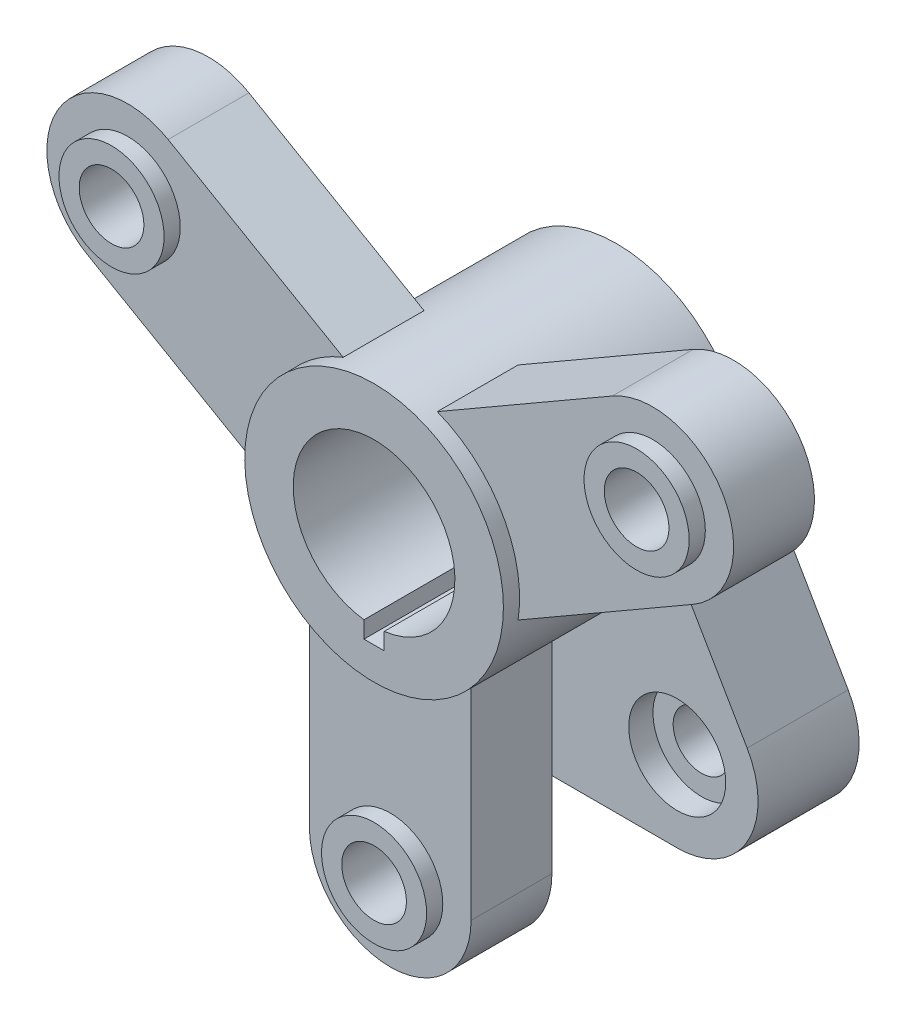
ISO-10303-21;
HEADER;
FILE_DESCRIPTION(('STEP AP214'),'2;1');
FILE_NAME('part.step','',(''),(''),'','','');
FILE_SCHEMA(('AUTOMOTIVE_DESIGN { 1 0 10303 214 1 1 1 1 }'));
ENDSEC;
DATA;
#1=APPLICATION_CONTEXT('core data for automotive mechanical design processes');
#2=APPLICATION_PROTOCOL_DEFINITION('international standard','automotive_design',2000,#1);
#3=PRODUCT_CONTEXT('',#1,'mechanical');
#4=PRODUCT('Part','Part','',(#3));
#5=PRODUCT_RELATED_PRODUCT_CATEGORY('part','',(#4));
#6=PRODUCT_DEFINITION_FORMATION('','',#4);
#7=PRODUCT_DEFINITION_CONTEXT('part definition',#1,'design');
#8=PRODUCT_DEFINITION('design','',#6,#7);
#9=PRODUCT_DEFINITION_SHAPE('','',#8);
#10=(LENGTH_UNIT() NAMED_UNIT(*) SI_UNIT(.MILLI.,.METRE.));
#11=(NAMED_UNIT(*) PLANE_ANGLE_UNIT() SI_UNIT($,.RADIAN.));
#12=(NAMED_UNIT(*) SI_UNIT($,.STERADIAN.) SOLID_ANGLE_UNIT());
#13=UNCERTAINTY_MEASURE_WITH_UNIT(LENGTH_MEASURE(1.E-05),#10,'distance_accuracy_value','');
#14=(GEOMETRIC_REPRESENTATION_CONTEXT(3) GLOBAL_UNCERTAINTY_ASSIGNED_CONTEXT((#13)) GLOBAL_UNIT_ASSIGNED_CONTEXT((#10,
#11,#12)) REPRESENTATION_CONTEXT('',''));
#15=CARTESIAN_POINT('',(0.,0.,0.));
#16=DIRECTION('',(0.,0.,1.));
#17=DIRECTION('',(1.,0.,0.));
#18=AXIS2_PLACEMENT_3D('',#15,#16,#17);
#19=CARTESIAN_POINT('',(0.,0.,56.));
#20=DIRECTION('',(0.,0.,1.));
#21=DIRECTION('',(1.,0.,0.));
#22=AXIS2_PLACEMENT_3D('',#19,#20,#21);
#23=PLANE('',#22);
#24=CARTESIAN_POINT('',(-64.951905283833,37.4999999999998,56.));
#25=DIRECTION('',(0.,0.,1.));
#26=DIRECTION('',(1.,0.,0.));
#27=AXIS2_PLACEMENT_3D('',#24,#25,#26);
#28=CIRCLE('',#27,13.);
#29=CARTESIAN_POINT('',(-51.951905283833,37.4999999999998,56.));
#30=VERTEX_POINT('',#29);
#31=EDGE_CURVE('E262',#30,#30,#28,.T.);
#32=ORIENTED_EDGE('',*,*,#31,.F.);
#33=EDGE_LOOP('',(#32));
#34=FACE_BOUND('',#33,.T.);
#35=CARTESIAN_POINT('',(0.,0.,56.));
#36=DIRECTION('',(0.,0.,1.));
#37=DIRECTION('',(1.,0.,0.));
#38=AXIS2_PLACEMENT_3D('',#35,#36,#37);
#39=CIRCLE('',#38,32.);
#40=CARTESIAN_POINT('',(-11.633307652784,29.8105040724855,56.));
#41=VERTEX_POINT('',#40);
#42=CARTESIAN_POINT('',(-31.6333076527839,-4.83051207889205,56.));
#43=VERTEX_POINT('',#42);
#44=EDGE_CURVE('E11',#41,#43,#39,.T.);
#45=ORIENTED_EDGE('',*,*,#44,.F.);
#46=DIRECTION('',(-0.86602540378444,0.499999999999998,0.));
#47=VECTOR('',#46,1.);
#48=CARTESIAN_POINT('',(-11.633307652784,29.8105040724855,56.));
#49=LINE('',#48,#47);
#50=CARTESIAN_POINT('',(-54.9519052838331,54.8205080756886,56.));
#51=VERTEX_POINT('',#50);
#52=EDGE_CURVE('E273',#41,#51,#49,.T.);
#53=ORIENTED_EDGE('',*,*,#52,.T.);
#54=CARTESIAN_POINT('',(-64.951905283833,37.4999999999998,56.));
#55=DIRECTION('',(0.,0.,1.));
#56=DIRECTION('',(1.,0.,0.));
#57=AXIS2_PLACEMENT_3D('',#54,#55,#56);
#58=CIRCLE('',#57,20.);
#59=CARTESIAN_POINT('',(-74.9519052838329,20.179491924311,56.));
#60=VERTEX_POINT('',#59);
#61=EDGE_CURVE('E295',#51,#60,#58,.T.);
#62=ORIENTED_EDGE('',*,*,#61,.T.);
#63=DIRECTION('',(0.86602540378444,-0.499999999999998,0.));
#64=VECTOR('',#63,1.);
#65=CARTESIAN_POINT('',(-31.6333076527839,-4.83051207889205,56.));
#66=LINE('',#65,#64);
#67=EDGE_CURVE('E278',#60,#43,#66,.T.);
#68=ORIENTED_EDGE('',*,*,#67,.T.);
#69=EDGE_LOOP('',(#45,#53,#62,#68));
#70=FACE_BOUND('',#69,.T.);
#71=ADVANCED_FACE('F50',(#34,#70),#23,.T.);
#72=CARTESIAN_POINT('',(0.,-75.,56.));
#73=DIRECTION('',(0.,0.,1.));
#74=DIRECTION('',(1.,0.,0.));
#75=AXIS2_PLACEMENT_3D('',#72,#73,#74);
#76=CIRCLE('',#75,13.);
#77=CARTESIAN_POINT('',(13.,-75.,56.));
#78=VERTEX_POINT('',#77);
#79=EDGE_CURVE('E255',#78,#78,#76,.T.);
#80=ORIENTED_EDGE('',*,*,#79,.F.);
#81=EDGE_LOOP('',(#80));
#82=FACE_BOUND('',#81,.T.);
#83=CARTESIAN_POINT('',(-20.,-24.9799919935936,56.));
#84=VERTEX_POINT('',#83);
#85=CARTESIAN_POINT('',(20.,-24.9799919935936,56.));
#86=VERTEX_POINT('',#85);
#87=EDGE_CURVE('E57',#84,#86,#39,.T.);
#88=ORIENTED_EDGE('',*,*,#87,.F.);
#89=DIRECTION('',(0.,-1.,0.));
#90=VECTOR('',#89,1.);
#91=CARTESIAN_POINT('',(-20.,-75.,56.));
#92=LINE('',#91,#90);
#93=CARTESIAN_POINT('',(-20.,-75.,56.));
#94=VERTEX_POINT('',#93);
#95=EDGE_CURVE('E297',#84,#94,#92,.T.);
#96=ORIENTED_EDGE('',*,*,#95,.T.);
#97=CARTESIAN_POINT('',(0.,-75.,56.));
#98=DIRECTION('',(0.,0.,1.));
#99=DIRECTION('',(1.,0.,0.));
#100=AXIS2_PLACEMENT_3D('',#97,#98,#99);
#101=CIRCLE('',#100,20.);
#102=CARTESIAN_POINT('',(20.,-75.,56.));
#103=VERTEX_POINT('',#102);
#104=EDGE_CURVE('E325',#94,#103,#101,.T.);
#105=ORIENTED_EDGE('',*,*,#104,.T.);
#106=DIRECTION('',(0.,1.,0.));
#107=VECTOR('',#106,1.);
#108=CARTESIAN_POINT('',(20.,-75.,56.));
#109=LINE('',#108,#107);
#110=EDGE_CURVE('E309',#103,#86,#109,.T.);
#111=ORIENTED_EDGE('',*,*,#110,.T.);
#112=EDGE_LOOP('',(#88,#96,#105,#111));
#113=FACE_BOUND('',#112,.T.);
#114=ADVANCED_FACE('F483',(#82,#113),#23,.T.);
#115=CARTESIAN_POINT('',(0.,-65.,25.));
#116=DIRECTION('',(0.,1.,0.));
#117=DIRECTION('',(0.,0.,1.));
#118=AXIS2_PLACEMENT_3D('',#115,#116,#117);
#119=PLANE('',#118);
#120=DIRECTION('',(1.,0.,0.));
#121=VECTOR('',#120,1.);
#122=CARTESIAN_POINT('',(0.,-65.,0.));
#123=LINE('',#122,#121);
#124=CARTESIAN_POINT('',(-40.,-65.,0.));
#125=VERTEX_POINT('',#124);
#126=CARTESIAN_POINT('',(40.,-65.,0.));
#127=VERTEX_POINT('',#126);
#128=EDGE_CURVE('E360',#125,#127,#123,.T.);
#129=ORIENTED_EDGE('',*,*,#128,.T.);
#130=DIRECTION('',(0.,0.,-1.));
#131=VECTOR('',#130,1.);
#132=CARTESIAN_POINT('',(40.,-65.,25.));
#133=LINE('',#132,#131);
#134=CARTESIAN_POINT('',(40.,-65.,25.));
#135=VERTEX_POINT('',#134);
#136=EDGE_CURVE('E366',#135,#127,#133,.T.);
#137=ORIENTED_EDGE('',*,*,#136,.F.);
#138=DIRECTION('',(1.,0.,0.));
#139=VECTOR('',#138,1.);
#140=CARTESIAN_POINT('',(0.,-65.,25.));
#141=LINE('',#140,#139);
#142=CARTESIAN_POINT('',(-40.,-65.,25.));
#143=VERTEX_POINT('',#142);
#144=EDGE_CURVE('E369',#143,#135,#141,.T.);
#145=ORIENTED_EDGE('',*,*,#144,.F.);
#146=DIRECTION('',(0.,0.,-1.));
#147=VECTOR('',#146,1.);
#148=CARTESIAN_POINT('',(-40.,-65.,25.));
#149=LINE('',#148,#147);
#150=EDGE_CURVE('E382',#143,#125,#149,.T.);
#151=ORIENTED_EDGE('',*,*,#150,.T.);
#152=EDGE_LOOP('',(#129,#137,#145,#151));
#153=FACE_BOUND('',#152,.T.);
#154=ADVANCED_FACE('F47',(#153),#119,.F.);
#155=CARTESIAN_POINT('',(40.,-45.,25.));
#156=DIRECTION('',(0.,0.,-1.));
#157=DIRECTION('',(-1.,0.,0.));
#158=AXIS2_PLACEMENT_3D('',#155,#156,#157);
#159=CYLINDRICAL_SURFACE('',#158,20.);
#160=CARTESIAN_POINT('',(40.,-45.,0.));
#161=DIRECTION('',(0.,0.,1.));
#162=DIRECTION('',(1.,0.,0.));
#163=AXIS2_PLACEMENT_3D('',#160,#161,#162);
#164=CIRCLE('',#163,20.);
#165=CARTESIAN_POINT('',(57.2965517241379,-34.9586206896552,0.));
#166=VERTEX_POINT('',#165);
#167=EDGE_CURVE('E387',#127,#166,#164,.T.);
#168=ORIENTED_EDGE('',*,*,#167,.T.);
#169=DIRECTION('',(0.,0.,-1.));
#170=VECTOR('',#169,1.);
#171=CARTESIAN_POINT('',(57.2965517241379,-34.9586206896552,25.));
#172=LINE('',#171,#170);
#173=CARTESIAN_POINT('',(57.2965517241379,-34.9586206896552,25.));
#174=VERTEX_POINT('',#173);
#175=EDGE_CURVE('E410',#174,#166,#172,.T.);
#176=ORIENTED_EDGE('',*,*,#175,.F.);
#177=CARTESIAN_POINT('',(40.,-45.,25.));
#178=DIRECTION('',(0.,0.,1.));
#179=DIRECTION('',(1.,0.,0.));
#180=AXIS2_PLACEMENT_3D('',#177,#178,#179);
#181=CIRCLE('',#180,20.);
#182=EDGE_CURVE('E375',#135,#174,#181,.T.);
#183=ORIENTED_EDGE('',*,*,#182,.F.);
#184=ORIENTED_EDGE('',*,*,#136,.T.);
#185=EDGE_LOOP('',(#168,#176,#183,#184));
#186=FACE_BOUND('',#185,.T.);
#187=ADVANCED_FACE('F467',(#186),#159,.T.);
#188=CARTESIAN_POINT('',(27.6744827586207,16.0662068965517,25.));
#189=DIRECTION('',(0.864827586206897,0.502068965517242,0.));
#190=DIRECTION('',(-0.502068965517242,0.864827586206897,0.));
#191=AXIS2_PLACEMENT_3D('',#188,#189,#190);
#192=PLANE('',#191);
#193=DIRECTION('',(0.502068965517242,-0.864827586206896,0.));
#194=VECTOR('',#193,1.);
#195=CARTESIAN_POINT('',(27.6744827586207,16.0662068965517,0.));
#196=LINE('',#195,#194);
#197=CARTESIAN_POINT('',(27.6744827586207,16.0662068965517,0.));
#198=VERTEX_POINT('',#197);
#199=EDGE_CURVE('E386',#198,#166,#196,.T.);
#200=ORIENTED_EDGE('',*,*,#199,.F.);
#201=DIRECTION('',(0.,0.,-1.));
#202=VECTOR('',#201,1.);
#203=CARTESIAN_POINT('',(27.6744827586207,16.0662068965517,25.));
#204=LINE('',#203,#202);
#205=CARTESIAN_POINT('',(27.6744827586207,16.0662068965517,25.));
#206=VERTEX_POINT('',#205);
#207=EDGE_CURVE('E403',#206,#198,#204,.T.);
#208=ORIENTED_EDGE('',*,*,#207,.F.);
#209=DIRECTION('',(0.502068965517242,-0.864827586206896,0.));
#210=VECTOR('',#209,1.);
#211=CARTESIAN_POINT('',(27.6744827586207,16.0662068965517,25.));
#212=LINE('',#211,#210);
#213=EDGE_CURVE('E374',#206,#174,#212,.T.);
#214=ORIENTED_EDGE('',*,*,#213,.T.);
#215=ORIENTED_EDGE('',*,*,#175,.T.);
#216=EDGE_LOOP('',(#200,#208,#214,#215));
#217=FACE_BOUND('',#216,.T.);
#218=ADVANCED_FACE('F466',(#217),#192,.T.);
#219=CARTESIAN_POINT('',(0.,0.,25.));
#220=DIRECTION('',(0.,0.,-1.));
#221=DIRECTION('',(-1.,0.,0.));
#222=AXIS2_PLACEMENT_3D('',#219,#220,#221);
#223=CYLINDRICAL_SURFACE('',#222,32.);
#224=DIRECTION('',(0.,0.,1.));
#225=VECTOR('',#224,1.);
#226=CARTESIAN_POINT('',(-11.633307652784,29.8105040724855,36.));
#227=LINE('',#226,#225);
#228=CARTESIAN_POINT('',(-11.633307652784,29.8105040724855,36.));
#229=VERTEX_POINT('',#228);
#230=EDGE_CURVE('E286',#229,#41,#227,.T.);
#231=ORIENTED_EDGE('',*,*,#230,.T.);
#232=ORIENTED_EDGE('',*,*,#44,.T.);
#233=DIRECTION('',(0.,0.,1.));
#234=VECTOR('',#233,1.);
#235=CARTESIAN_POINT('',(-31.6333076527839,-4.83051207889205,36.));
#236=LINE('',#235,#234);
#237=CARTESIAN_POINT('',(-31.6333076527839,-4.83051207889205,36.));
#238=VERTEX_POINT('',#237);
#239=EDGE_CURVE('E298',#238,#43,#236,.T.);
#240=ORIENTED_EDGE('',*,*,#239,.F.);
#241=CARTESIAN_POINT('',(0.,0.,36.));
#242=DIRECTION('',(0.,0.,-1.));
#243=DIRECTION('',(1.,0.,0.));
#244=AXIS2_PLACEMENT_3D('',#241,#242,#243);
#245=CIRCLE('',#244,32.);
#246=EDGE_CURVE('E277',#238,#229,#245,.T.);
#247=ORIENTED_EDGE('',*,*,#246,.T.);
#248=EDGE_LOOP('',(#231,#232,#240,#247));
#249=FACE_BOUND('',#248,.T.);
#250=DIRECTION('',(0.,0.,1.));
#251=VECTOR('',#250,1.);
#252=CARTESIAN_POINT('',(-20.,-24.9799919935936,36.));
#253=LINE('',#252,#251);
#254=CARTESIAN_POINT('',(-20.,-24.9799919935936,36.));
#255=VERTEX_POINT('',#254);
#256=EDGE_CURVE('E317',#255,#84,#253,.T.);
#257=ORIENTED_EDGE('',*,*,#256,.T.);
#258=ORIENTED_EDGE('',*,*,#87,.T.);
#259=DIRECTION('',(0.,0.,1.));
#260=VECTOR('',#259,1.);
#261=CARTESIAN_POINT('',(20.,-24.9799919935936,36.));
#262=LINE('',#261,#260);
#263=CARTESIAN_POINT('',(20.,-24.9799919935936,36.));
#264=VERTEX_POINT('',#263);
#265=EDGE_CURVE('E326',#264,#86,#262,.T.);
#266=ORIENTED_EDGE('',*,*,#265,.F.);
#267=CARTESIAN_POINT('',(0.,0.,36.));
#268=DIRECTION('',(0.,0.,-1.));
#269=DIRECTION('',(1.,0.,0.));
#270=AXIS2_PLACEMENT_3D('',#267,#268,#269);
#271=CIRCLE('',#270,32.);
#272=EDGE_CURVE('E308',#264,#255,#271,.T.);
#273=ORIENTED_EDGE('',*,*,#272,.T.);
#274=EDGE_LOOP('',(#257,#258,#266,#273));
#275=FACE_BOUND('',#274,.T.);
#276=CARTESIAN_POINT('',(31.6314798513526,-4.84246656296924,56.));
#277=VERTEX_POINT('',#276);
#278=CARTESIAN_POINT('',(11.633307652784,29.8105040724856,56.));
#279=VERTEX_POINT('',#278);
#280=EDGE_CURVE('E59',#277,#279,#39,.T.);
#281=ORIENTED_EDGE('',*,*,#280,.T.);
#282=DIRECTION('',(0.,0.,1.));
#283=VECTOR('',#282,1.);
#284=CARTESIAN_POINT('',(11.633307652784,29.8105040724856,36.));
#285=LINE('',#284,#283);
#286=CARTESIAN_POINT('',(11.633307652784,29.8105040724856,36.));
#287=VERTEX_POINT('',#286);
#288=EDGE_CURVE('E354',#287,#279,#285,.T.);
#289=ORIENTED_EDGE('',*,*,#288,.F.);
#290=CARTESIAN_POINT('',(0.,0.,36.));
#291=DIRECTION('',(0.,0.,-1.));
#292=DIRECTION('',(1.,0.,0.));
#293=AXIS2_PLACEMENT_3D('',#290,#291,#292);
#294=CIRCLE('',#293,32.);
#295=CARTESIAN_POINT('',(31.6314798513526,-4.84246656296924,36.));
#296=VERTEX_POINT('',#295);
#297=EDGE_CURVE('E338',#287,#296,#294,.T.);
#298=ORIENTED_EDGE('',*,*,#297,.T.);
#299=DIRECTION('',(0.,0.,1.));
#300=VECTOR('',#299,1.);
#301=CARTESIAN_POINT('',(31.6314798513526,-4.84246656296924,36.));
#302=LINE('',#301,#300);
#303=EDGE_CURVE('E350',#296,#277,#302,.T.);
#304=ORIENTED_EDGE('',*,*,#303,.T.);
#305=EDGE_LOOP('',(#281,#289,#298,#304));
#306=FACE_BOUND('',#305,.T.);
#307=CARTESIAN_POINT('',(0.,0.,0.));
#308=DIRECTION('',(0.,0.,1.));
#309=DIRECTION('',(1.,0.,0.));
#310=AXIS2_PLACEMENT_3D('',#307,#308,#309);
#311=CIRCLE('',#310,32.);
#312=CARTESIAN_POINT('',(-27.6744827586207,16.0662068965517,0.));
#313=VERTEX_POINT('',#312);
#314=EDGE_CURVE('E395',#198,#313,#311,.T.);
#315=ORIENTED_EDGE('',*,*,#314,.T.);
#316=DIRECTION('',(0.,0.,-1.));
#317=VECTOR('',#316,1.);
#318=CARTESIAN_POINT('',(-27.6744827586207,16.0662068965517,25.));
#319=LINE('',#318,#317);
#320=CARTESIAN_POINT('',(-27.6744827586207,16.0662068965517,25.));
#321=VERTEX_POINT('',#320);
#322=EDGE_CURVE('E401',#321,#313,#319,.T.);
#323=ORIENTED_EDGE('',*,*,#322,.F.);
#324=CARTESIAN_POINT('',(0.,0.,25.));
#325=DIRECTION('',(0.,0.,1.));
#326=DIRECTION('',(1.,0.,0.));
#327=AXIS2_PLACEMENT_3D('',#324,#325,#326);
#328=CIRCLE('',#327,32.);
#329=EDGE_CURVE('E364',#321,#206,#328,.T.);
#330=ORIENTED_EDGE('',*,*,#329,.T.);
#331=ORIENTED_EDGE('',*,*,#207,.T.);
#332=EDGE_LOOP('',(#315,#323,#330,#331));
#333=FACE_BOUND('',#332,.T.);
#334=CARTESIAN_POINT('',(0.,0.,60.));
#335=DIRECTION('',(0.,0.,1.));
#336=DIRECTION('',(1.,0.,0.));
#337=AXIS2_PLACEMENT_3D('',#334,#335,#336);
#338=CIRCLE('',#337,32.);
#339=CARTESIAN_POINT('',(32.,0.,60.));
#340=VERTEX_POINT('',#339);
#341=EDGE_CURVE('E269',#340,#340,#338,.T.);
#342=ORIENTED_EDGE('',*,*,#341,.F.);
#343=EDGE_LOOP('',(#342));
#344=FACE_BOUND('',#343,.T.);
#345=ADVANCED_FACE('F449',(#249,#275,#306,#333,#344),#223,.T.);
#346=CARTESIAN_POINT('',(-27.6744827586207,16.0662068965517,25.));
#347=DIRECTION('',(-0.864827586206897,0.502068965517241,0.));
#348=DIRECTION('',(-0.502068965517241,-0.864827586206897,0.));
#349=AXIS2_PLACEMENT_3D('',#346,#347,#348);
#350=PLANE('',#349);
#351=DIRECTION('',(0.502068965517241,0.864827586206897,0.));
#352=VECTOR('',#351,1.);
#353=CARTESIAN_POINT('',(-27.6744827586207,16.0662068965517,0.));
#354=LINE('',#353,#352);
#355=CARTESIAN_POINT('',(-57.2965517241379,-34.9586206896552,0.));
#356=VERTEX_POINT('',#355);
#357=EDGE_CURVE('E394',#356,#313,#354,.T.);
#358=ORIENTED_EDGE('',*,*,#357,.F.);
#359=DIRECTION('',(0.,0.,-1.));
#360=VECTOR('',#359,1.);
#361=CARTESIAN_POINT('',(-57.2965517241379,-34.9586206896552,25.));
#362=LINE('',#361,#360);
#363=CARTESIAN_POINT('',(-57.2965517241379,-34.9586206896552,25.));
#364=VERTEX_POINT('',#363);
#365=EDGE_CURVE('E402',#364,#356,#362,.T.);
#366=ORIENTED_EDGE('',*,*,#365,.F.);
#367=DIRECTION('',(0.502068965517241,0.864827586206897,0.));
#368=VECTOR('',#367,1.);
#369=CARTESIAN_POINT('',(-27.6744827586207,16.0662068965517,25.));
#370=LINE('',#369,#368);
#371=EDGE_CURVE('E378',#364,#321,#370,.T.);
#372=ORIENTED_EDGE('',*,*,#371,.T.);
#373=ORIENTED_EDGE('',*,*,#322,.T.);
#374=EDGE_LOOP('',(#358,#366,#372,#373));
#375=FACE_BOUND('',#374,.T.);
#376=ADVANCED_FACE('F453',(#375),#350,.T.);
#377=CARTESIAN_POINT('',(-40.,-45.,25.));
#378=DIRECTION('',(0.,0.,-1.));
#379=DIRECTION('',(-1.,0.,0.));
#380=AXIS2_PLACEMENT_3D('',#377,#378,#379);
#381=CYLINDRICAL_SURFACE('',#380,20.);
#382=CARTESIAN_POINT('',(-40.,-45.,0.));
#383=DIRECTION('',(0.,0.,1.));
#384=DIRECTION('',(1.,0.,0.));
#385=AXIS2_PLACEMENT_3D('',#382,#383,#384);
#386=CIRCLE('',#385,20.);
#387=EDGE_CURVE('E373',#356,#125,#386,.T.);
#388=ORIENTED_EDGE('',*,*,#387,.T.);
#389=ORIENTED_EDGE('',*,*,#150,.F.);
#390=CARTESIAN_POINT('',(-40.,-45.,25.));
#391=DIRECTION('',(0.,0.,1.));
#392=DIRECTION('',(1.,0.,0.));
#393=AXIS2_PLACEMENT_3D('',#390,#391,#392);
#394=CIRCLE('',#393,20.);
#395=EDGE_CURVE('E381',#364,#143,#394,.T.);
#396=ORIENTED_EDGE('',*,*,#395,.F.);
#397=ORIENTED_EDGE('',*,*,#365,.T.);
#398=EDGE_LOOP('',(#388,#389,#396,#397));
#399=FACE_BOUND('',#398,.T.);
#400=ADVANCED_FACE('F444',(#399),#381,.T.);
#401=CARTESIAN_POINT('',(0.,0.,25.));
#402=DIRECTION('',(0.,0.,1.));
#403=DIRECTION('',(1.,0.,0.));
#404=AXIS2_PLACEMENT_3D('',#401,#402,#403);
#405=PLANE('',#404);
#406=CARTESIAN_POINT('',(-40.,-45.,25.));
#407=DIRECTION('',(0.,0.,1.));
#408=DIRECTION('',(1.,0.,0.));
#409=AXIS2_PLACEMENT_3D('',#406,#407,#408);
#410=CIRCLE('',#409,12.);
#411=CARTESIAN_POINT('',(-28.,-45.,25.));
#412=VERTEX_POINT('',#411);
#413=EDGE_CURVE('E428',#412,#412,#410,.T.);
#414=ORIENTED_EDGE('',*,*,#413,.F.);
#415=EDGE_LOOP('',(#414));
#416=FACE_BOUND('',#415,.T.);
#417=CARTESIAN_POINT('',(40.,-45.,25.));
#418=DIRECTION('',(0.,0.,1.));
#419=DIRECTION('',(1.,0.,0.));
#420=AXIS2_PLACEMENT_3D('',#417,#418,#419);
#421=CIRCLE('',#420,12.);
#422=CARTESIAN_POINT('',(52.,-45.,25.));
#423=VERTEX_POINT('',#422);
#424=EDGE_CURVE('E418',#423,#423,#421,.T.);
#425=ORIENTED_EDGE('',*,*,#424,.F.);
#426=EDGE_LOOP('',(#425));
#427=FACE_BOUND('',#426,.T.);
#428=ORIENTED_EDGE('',*,*,#329,.F.);
#429=ORIENTED_EDGE('',*,*,#371,.F.);
#430=ORIENTED_EDGE('',*,*,#395,.T.);
#431=ORIENTED_EDGE('',*,*,#144,.T.);
#432=ORIENTED_EDGE('',*,*,#182,.T.);
#433=ORIENTED_EDGE('',*,*,#213,.F.);
#434=EDGE_LOOP('',(#428,#429,#430,#431,#432,#433));
#435=FACE_BOUND('',#434,.T.);
#436=ADVANCED_FACE('F438',(#416,#427,#435),#405,.T.);
#437=CARTESIAN_POINT('',(0.,0.,0.));
#438=DIRECTION('',(0.,0.,1.));
#439=DIRECTION('',(1.,0.,0.));
#440=AXIS2_PLACEMENT_3D('',#437,#438,#439);
#441=PLANE('',#440);
#442=CARTESIAN_POINT('',(-40.,-45.,0.));
#443=DIRECTION('',(0.,0.,1.));
#444=DIRECTION('',(1.,0.,0.));
#445=AXIS2_PLACEMENT_3D('',#442,#443,#444);
#446=CIRCLE('',#445,7.);
#447=CARTESIAN_POINT('',(-33.,-45.,0.));
#448=VERTEX_POINT('',#447);
#449=EDGE_CURVE('E51',#448,#448,#446,.T.);
#450=ORIENTED_EDGE('',*,*,#449,.T.);
#451=EDGE_LOOP('',(#450));
#452=FACE_BOUND('',#451,.T.);
#453=CARTESIAN_POINT('',(40.,-45.,0.));
#454=DIRECTION('',(0.,0.,1.));
#455=DIRECTION('',(1.,0.,0.));
#456=AXIS2_PLACEMENT_3D('',#453,#454,#455);
#457=CIRCLE('',#456,7.);
#458=CARTESIAN_POINT('',(47.,-45.,0.));
#459=VERTEX_POINT('',#458);
#460=EDGE_CURVE('E409',#459,#459,#457,.T.);
#461=ORIENTED_EDGE('',*,*,#460,.T.);
#462=EDGE_LOOP('',(#461));
#463=FACE_BOUND('',#462,.T.);
#464=DIRECTION('',(1.,0.,0.));
#465=VECTOR('',#464,1.);
#466=CARTESIAN_POINT('',(0.,-24.,0.));
#467=LINE('',#466,#465);
#468=CARTESIAN_POINT('',(-2.5,-24.,0.));
#469=VERTEX_POINT('',#468);
#470=CARTESIAN_POINT('',(2.5,-24.,0.));
#471=VERTEX_POINT('',#470);
#472=EDGE_CURVE('E229',#469,#471,#467,.T.);
#473=ORIENTED_EDGE('',*,*,#472,.T.);
#474=DIRECTION('',(0.,1.,0.));
#475=VECTOR('',#474,1.);
#476=CARTESIAN_POINT('',(2.5,0.,0.));
#477=LINE('',#476,#475);
#478=CARTESIAN_POINT('',(2.5,-19.8431348329844,0.));
#479=VERTEX_POINT('',#478);
#480=EDGE_CURVE('E234',#471,#479,#477,.T.);
#481=ORIENTED_EDGE('',*,*,#480,.T.);
#482=CARTESIAN_POINT('',(0.,0.,0.));
#483=DIRECTION('',(0.,0.,1.));
#484=DIRECTION('',(1.,0.,0.));
#485=AXIS2_PLACEMENT_3D('',#482,#483,#484);
#486=CIRCLE('',#485,20.);
#487=CARTESIAN_POINT('',(-2.5,-19.8431348329844,0.));
#488=VERTEX_POINT('',#487);
#489=EDGE_CURVE('E223',#479,#488,#486,.T.);
#490=ORIENTED_EDGE('',*,*,#489,.T.);
#491=DIRECTION('',(0.,-1.,0.));
#492=VECTOR('',#491,1.);
#493=CARTESIAN_POINT('',(-2.5,0.,0.));
#494=LINE('',#493,#492);
#495=EDGE_CURVE('E202',#488,#469,#494,.T.);
#496=ORIENTED_EDGE('',*,*,#495,.T.);
#497=EDGE_LOOP('',(#473,#481,#490,#496));
#498=FACE_BOUND('',#497,.T.);
#499=ORIENTED_EDGE('',*,*,#128,.F.);
#500=ORIENTED_EDGE('',*,*,#387,.F.);
#501=ORIENTED_EDGE('',*,*,#357,.T.);
#502=ORIENTED_EDGE('',*,*,#314,.F.);
#503=ORIENTED_EDGE('',*,*,#199,.T.);
#504=ORIENTED_EDGE('',*,*,#167,.F.);
#505=EDGE_LOOP('',(#499,#500,#501,#502,#503,#504));
#506=FACE_BOUND('',#505,.T.);
#507=ADVANCED_FACE('F445',(#452,#463,#498,#506),#441,.F.);
#508=CARTESIAN_POINT('',(64.951905283833,37.4999999999997,56.));
#509=DIRECTION('',(0.,0.,1.));
#510=DIRECTION('',(1.,0.,0.));
#511=AXIS2_PLACEMENT_3D('',#508,#509,#510);
#512=CIRCLE('',#511,13.);
#513=CARTESIAN_POINT('',(77.951905283833,37.4999999999997,56.));
#514=VERTEX_POINT('',#513);
#515=EDGE_CURVE('E256',#514,#514,#512,.T.);
#516=ORIENTED_EDGE('',*,*,#515,.F.);
#517=EDGE_LOOP('',(#516));
#518=FACE_BOUND('',#517,.T.);
#519=ORIENTED_EDGE('',*,*,#280,.F.);
#520=DIRECTION('',(0.865931054082888,0.500163382880933,0.));
#521=VECTOR('',#520,1.);
#522=CARTESIAN_POINT('',(37.7583689317868,-1.3035640665669,56.));
#523=LINE('',#522,#521);
#524=CARTESIAN_POINT('',(74.9551729414516,20.1813789183421,56.));
#525=VERTEX_POINT('',#524);
#526=EDGE_CURVE('E328',#277,#525,#523,.T.);
#527=ORIENTED_EDGE('',*,*,#526,.T.);
#528=CARTESIAN_POINT('',(64.951905283833,37.4999999999997,56.));
#529=DIRECTION('',(0.,0.,1.));
#530=DIRECTION('',(1.,0.,0.));
#531=AXIS2_PLACEMENT_3D('',#528,#529,#530);
#532=CIRCLE('',#531,19.9999999999999);
#533=CARTESIAN_POINT('',(54.9519052838332,54.8205080756884,56.));
#534=VERTEX_POINT('',#533);
#535=EDGE_CURVE('E348',#525,#534,#532,.T.);
#536=ORIENTED_EDGE('',*,*,#535,.T.);
#537=DIRECTION('',(-0.866025403784444,-0.499999999999991,0.));
#538=VECTOR('',#537,1.);
#539=CARTESIAN_POINT('',(17.2807388545969,33.0710499970821,56.));
#540=LINE('',#539,#538);
#541=EDGE_CURVE('E339',#534,#279,#540,.T.);
#542=ORIENTED_EDGE('',*,*,#541,.T.);
#543=EDGE_LOOP('',(#519,#527,#536,#542));
#544=FACE_BOUND('',#543,.T.);
#545=ADVANCED_FACE('F472',(#518,#544),#23,.T.);
#546=CARTESIAN_POINT('',(17.2807388545969,33.0710499970821,36.));
#547=DIRECTION('',(-0.499999999999991,0.866025403784444,0.));
#548=DIRECTION('',(-0.866025403784444,-0.499999999999991,0.));
#549=AXIS2_PLACEMENT_3D('',#546,#547,#548);
#550=PLANE('',#549);
#551=ORIENTED_EDGE('',*,*,#541,.F.);
#552=DIRECTION('',(0.,0.,1.));
#553=VECTOR('',#552,1.);
#554=CARTESIAN_POINT('',(54.9519052838332,54.8205080756884,36.));
#555=LINE('',#554,#553);
#556=CARTESIAN_POINT('',(54.9519052838332,54.8205080756884,36.));
#557=VERTEX_POINT('',#556);
#558=EDGE_CURVE('E359',#557,#534,#555,.T.);
#559=ORIENTED_EDGE('',*,*,#558,.F.);
#560=DIRECTION('',(-0.866025403784443,-0.499999999999993,0.));
#561=VECTOR('',#560,1.);
#562=CARTESIAN_POINT('',(17.2807388545969,33.0710499970821,36.));
#563=LINE('',#562,#561);
#564=EDGE_CURVE('E343',#557,#287,#563,.T.);
#565=ORIENTED_EDGE('',*,*,#564,.T.);
#566=ORIENTED_EDGE('',*,*,#288,.T.);
#567=EDGE_LOOP('',(#551,#559,#565,#566));
#568=FACE_BOUND('',#567,.T.);
#569=ADVANCED_FACE('F477',(#568),#550,.T.);
#570=CARTESIAN_POINT('',(64.951905283833,37.4999999999997,36.));
#571=DIRECTION('',(0.,0.,1.));
#572=DIRECTION('',(1.,0.,0.));
#573=AXIS2_PLACEMENT_3D('',#570,#571,#572);
#574=CYLINDRICAL_SURFACE('',#573,19.9999999999999);
#575=ORIENTED_EDGE('',*,*,#535,.F.);
#576=DIRECTION('',(0.,0.,1.));
#577=VECTOR('',#576,1.);
#578=CARTESIAN_POINT('',(74.9551729414516,20.1813789183421,36.));
#579=LINE('',#578,#577);
#580=CARTESIAN_POINT('',(74.9551729414516,20.1813789183421,36.));
#581=VERTEX_POINT('',#580);
#582=EDGE_CURVE('E363',#581,#525,#579,.T.);
#583=ORIENTED_EDGE('',*,*,#582,.F.);
#584=CARTESIAN_POINT('',(64.951905283833,37.4999999999997,36.));
#585=DIRECTION('',(0.,0.,1.));
#586=DIRECTION('',(1.,0.,0.));
#587=AXIS2_PLACEMENT_3D('',#584,#585,#586);
#588=CIRCLE('',#587,19.9999999999999);
#589=EDGE_CURVE('E345',#581,#557,#588,.T.);
#590=ORIENTED_EDGE('',*,*,#589,.T.);
#591=ORIENTED_EDGE('',*,*,#558,.T.);
#592=EDGE_LOOP('',(#575,#583,#590,#591));
#593=FACE_BOUND('',#592,.T.);
#594=ADVANCED_FACE('F496',(#593),#574,.T.);
#595=CARTESIAN_POINT('',(37.7583689317868,-1.3035640665669,36.));
#596=DIRECTION('',(0.500163382880933,-0.865931054082888,0.));
#597=DIRECTION('',(0.865931054082888,0.500163382880933,0.));
#598=AXIS2_PLACEMENT_3D('',#595,#596,#597);
#599=PLANE('',#598);
#600=ORIENTED_EDGE('',*,*,#526,.F.);
#601=ORIENTED_EDGE('',*,*,#303,.F.);
#602=DIRECTION('',(0.865931054082888,0.500163382880933,0.));
#603=VECTOR('',#602,1.);
#604=CARTESIAN_POINT('',(37.7583689317868,-1.3035640665669,36.));
#605=LINE('',#604,#603);
#606=EDGE_CURVE('E337',#296,#581,#605,.T.);
#607=ORIENTED_EDGE('',*,*,#606,.T.);
#608=ORIENTED_EDGE('',*,*,#582,.T.);
#609=EDGE_LOOP('',(#600,#601,#607,#608));
#610=FACE_BOUND('',#609,.T.);
#611=ADVANCED_FACE('F494',(#610),#599,.T.);
#612=CARTESIAN_POINT('',(0.,0.,36.));
#613=DIRECTION('',(0.,0.,1.));
#614=DIRECTION('',(1.,0.,0.));
#615=AXIS2_PLACEMENT_3D('',#612,#613,#614);
#616=PLANE('',#615);
#617=CARTESIAN_POINT('',(64.951905283833,37.4999999999997,36.));
#618=DIRECTION('',(0.,0.,1.));
#619=DIRECTION('',(1.,0.,0.));
#620=AXIS2_PLACEMENT_3D('',#617,#618,#619);
#621=CIRCLE('',#620,8.00000000000001);
#622=CARTESIAN_POINT('',(72.951905283833,37.4999999999997,36.));
#623=VERTEX_POINT('',#622);
#624=EDGE_CURVE('E249',#623,#623,#621,.T.);
#625=ORIENTED_EDGE('',*,*,#624,.T.);
#626=EDGE_LOOP('',(#625));
#627=FACE_BOUND('',#626,.T.);
#628=ORIENTED_EDGE('',*,*,#297,.F.);
#629=ORIENTED_EDGE('',*,*,#564,.F.);
#630=ORIENTED_EDGE('',*,*,#589,.F.);
#631=ORIENTED_EDGE('',*,*,#606,.F.);
#632=EDGE_LOOP('',(#628,#629,#630,#631));
#633=FACE_BOUND('',#632,.T.);
#634=ADVANCED_FACE('F499',(#627,#633),#616,.F.);
#635=CARTESIAN_POINT('',(20.,-75.,36.));
#636=DIRECTION('',(1.,0.,0.));
#637=DIRECTION('',(0.,0.,-1.));
#638=AXIS2_PLACEMENT_3D('',#635,#636,#637);
#639=PLANE('',#638);
#640=ORIENTED_EDGE('',*,*,#110,.F.);
#641=DIRECTION('',(0.,0.,1.));
#642=VECTOR('',#641,1.);
#643=CARTESIAN_POINT('',(20.,-75.,36.));
#644=LINE('',#643,#642);
#645=CARTESIAN_POINT('',(20.,-75.,36.));
#646=VERTEX_POINT('',#645);
#647=EDGE_CURVE('E329',#646,#103,#644,.T.);
#648=ORIENTED_EDGE('',*,*,#647,.F.);
#649=DIRECTION('',(0.,1.,0.));
#650=VECTOR('',#649,1.);
#651=CARTESIAN_POINT('',(20.,-75.,36.));
#652=LINE('',#651,#650);
#653=EDGE_CURVE('E316',#646,#264,#652,.T.);
#654=ORIENTED_EDGE('',*,*,#653,.T.);
#655=ORIENTED_EDGE('',*,*,#265,.T.);
#656=EDGE_LOOP('',(#640,#648,#654,#655));
#657=FACE_BOUND('',#656,.T.);
#658=ADVANCED_FACE('F506',(#657),#639,.T.);
#659=CARTESIAN_POINT('',(0.,-75.,36.));
#660=DIRECTION('',(0.,0.,1.));
#661=DIRECTION('',(1.,0.,0.));
#662=AXIS2_PLACEMENT_3D('',#659,#660,#661);
#663=CYLINDRICAL_SURFACE('',#662,20.);
#664=ORIENTED_EDGE('',*,*,#104,.F.);
#665=DIRECTION('',(0.,0.,1.));
#666=VECTOR('',#665,1.);
#667=CARTESIAN_POINT('',(-20.,-75.,36.));
#668=LINE('',#667,#666);
#669=CARTESIAN_POINT('',(-20.,-75.,36.));
#670=VERTEX_POINT('',#669);
#671=EDGE_CURVE('E335',#670,#94,#668,.T.);
#672=ORIENTED_EDGE('',*,*,#671,.F.);
#673=CARTESIAN_POINT('',(0.,-75.,36.));
#674=DIRECTION('',(0.,0.,1.));
#675=DIRECTION('',(1.,0.,0.));
#676=AXIS2_PLACEMENT_3D('',#673,#674,#675);
#677=CIRCLE('',#676,20.);
#678=EDGE_CURVE('E311',#670,#646,#677,.T.);
#679=ORIENTED_EDGE('',*,*,#678,.T.);
#680=ORIENTED_EDGE('',*,*,#647,.T.);
#681=EDGE_LOOP('',(#664,#672,#679,#680));
#682=FACE_BOUND('',#681,.T.);
#683=ADVANCED_FACE('F513',(#682),#663,.T.);
#684=CARTESIAN_POINT('',(-20.,-75.,36.));
#685=DIRECTION('',(-1.,0.,0.));
#686=DIRECTION('',(0.,0.,1.));
#687=AXIS2_PLACEMENT_3D('',#684,#685,#686);
#688=PLANE('',#687);
#689=ORIENTED_EDGE('',*,*,#95,.F.);
#690=ORIENTED_EDGE('',*,*,#256,.F.);
#691=DIRECTION('',(0.,-1.,0.));
#692=VECTOR('',#691,1.);
#693=CARTESIAN_POINT('',(-20.,-75.,36.));
#694=LINE('',#693,#692);
#695=EDGE_CURVE('E310',#255,#670,#694,.T.);
#696=ORIENTED_EDGE('',*,*,#695,.T.);
#697=ORIENTED_EDGE('',*,*,#671,.T.);
#698=EDGE_LOOP('',(#689,#690,#696,#697));
#699=FACE_BOUND('',#698,.T.);
#700=ADVANCED_FACE('F512',(#699),#688,.T.);
#701=CARTESIAN_POINT('',(0.,0.,36.));
#702=DIRECTION('',(0.,0.,1.));
#703=DIRECTION('',(1.,0.,0.));
#704=AXIS2_PLACEMENT_3D('',#701,#702,#703);
#705=PLANE('',#704);
#706=CARTESIAN_POINT('',(0.,-75.,36.));
#707=DIRECTION('',(0.,0.,1.));
#708=DIRECTION('',(1.,0.,0.));
#709=AXIS2_PLACEMENT_3D('',#706,#707,#708);
#710=CIRCLE('',#709,8.);
#711=CARTESIAN_POINT('',(8.,-75.,36.));
#712=VERTEX_POINT('',#711);
#713=EDGE_CURVE('E238',#712,#712,#710,.T.);
#714=ORIENTED_EDGE('',*,*,#713,.T.);
#715=EDGE_LOOP('',(#714));
#716=FACE_BOUND('',#715,.T.);
#717=ORIENTED_EDGE('',*,*,#272,.F.);
#718=ORIENTED_EDGE('',*,*,#653,.F.);
#719=ORIENTED_EDGE('',*,*,#678,.F.);
#720=ORIENTED_EDGE('',*,*,#695,.F.);
#721=EDGE_LOOP('',(#717,#718,#719,#720));
#722=FACE_BOUND('',#721,.T.);
#723=ADVANCED_FACE('F514',(#716,#722),#705,.F.);
#724=CARTESIAN_POINT('',(-31.6333076527839,-4.83051207889205,36.));
#725=DIRECTION('',(-0.499999999999998,-0.86602540378444,0.));
#726=DIRECTION('',(0.86602540378444,-0.499999999999998,0.));
#727=AXIS2_PLACEMENT_3D('',#724,#725,#726);
#728=PLANE('',#727);
#729=ORIENTED_EDGE('',*,*,#67,.F.);
#730=DIRECTION('',(0.,0.,1.));
#731=VECTOR('',#730,1.);
#732=CARTESIAN_POINT('',(-74.9519052838329,20.179491924311,36.));
#733=LINE('',#732,#731);
#734=CARTESIAN_POINT('',(-74.9519052838329,20.179491924311,36.));
#735=VERTEX_POINT('',#734);
#736=EDGE_CURVE('E299',#735,#60,#733,.T.);
#737=ORIENTED_EDGE('',*,*,#736,.F.);
#738=DIRECTION('',(0.86602540378444,-0.499999999999998,0.));
#739=VECTOR('',#738,1.);
#740=CARTESIAN_POINT('',(-31.6333076527839,-4.83051207889205,36.));
#741=LINE('',#740,#739);
#742=EDGE_CURVE('E287',#735,#238,#741,.T.);
#743=ORIENTED_EDGE('',*,*,#742,.T.);
#744=ORIENTED_EDGE('',*,*,#239,.T.);
#745=EDGE_LOOP('',(#729,#737,#743,#744));
#746=FACE_BOUND('',#745,.T.);
#747=ADVANCED_FACE('F523',(#746),#728,.T.);
#748=CARTESIAN_POINT('',(-64.951905283833,37.4999999999998,36.));
#749=DIRECTION('',(0.,0.,1.));
#750=DIRECTION('',(1.,0.,0.));
#751=AXIS2_PLACEMENT_3D('',#748,#749,#750);
#752=CYLINDRICAL_SURFACE('',#751,20.);
#753=ORIENTED_EDGE('',*,*,#61,.F.);
#754=DIRECTION('',(0.,0.,1.));
#755=VECTOR('',#754,1.);
#756=CARTESIAN_POINT('',(-54.9519052838331,54.8205080756886,36.));
#757=LINE('',#756,#755);
#758=CARTESIAN_POINT('',(-54.9519052838331,54.8205080756886,36.));
#759=VERTEX_POINT('',#758);
#760=EDGE_CURVE('E305',#759,#51,#757,.T.);
#761=ORIENTED_EDGE('',*,*,#760,.F.);
#762=CARTESIAN_POINT('',(-64.951905283833,37.4999999999998,36.));
#763=DIRECTION('',(0.,0.,1.));
#764=DIRECTION('',(1.,0.,0.));
#765=AXIS2_PLACEMENT_3D('',#762,#763,#764);
#766=CIRCLE('',#765,20.);
#767=EDGE_CURVE('E281',#759,#735,#766,.T.);
#768=ORIENTED_EDGE('',*,*,#767,.T.);
#769=ORIENTED_EDGE('',*,*,#736,.T.);
#770=EDGE_LOOP('',(#753,#761,#768,#769));
#771=FACE_BOUND('',#770,.T.);
#772=ADVANCED_FACE('F529',(#771),#752,.T.);
#773=CARTESIAN_POINT('',(-11.633307652784,29.8105040724855,36.));
#774=DIRECTION('',(0.499999999999998,0.86602540378444,0.));
#775=DIRECTION('',(-0.86602540378444,0.499999999999998,0.));
#776=AXIS2_PLACEMENT_3D('',#773,#774,#775);
#777=PLANE('',#776);
#778=ORIENTED_EDGE('',*,*,#52,.F.);
#779=ORIENTED_EDGE('',*,*,#230,.F.);
#780=DIRECTION('',(-0.86602540378444,0.499999999999998,0.));
#781=VECTOR('',#780,1.);
#782=CARTESIAN_POINT('',(-11.633307652784,29.8105040724855,36.));
#783=LINE('',#782,#781);
#784=EDGE_CURVE('E276',#229,#759,#783,.T.);
#785=ORIENTED_EDGE('',*,*,#784,.T.);
#786=ORIENTED_EDGE('',*,*,#760,.T.);
#787=EDGE_LOOP('',(#778,#779,#785,#786));
#788=FACE_BOUND('',#787,.T.);
#789=ADVANCED_FACE('F527',(#788),#777,.T.);
#790=CARTESIAN_POINT('',(0.,0.,36.));
#791=DIRECTION('',(0.,0.,1.));
#792=DIRECTION('',(1.,0.,0.));
#793=AXIS2_PLACEMENT_3D('',#790,#791,#792);
#794=PLANE('',#793);
#795=CARTESIAN_POINT('',(-64.951905283833,37.4999999999998,36.));
#796=DIRECTION('',(0.,0.,1.));
#797=DIRECTION('',(1.,0.,0.));
#798=AXIS2_PLACEMENT_3D('',#795,#796,#797);
#799=CIRCLE('',#798,8.00000000000001);
#800=CARTESIAN_POINT('',(-56.951905283833,37.4999999999998,36.));
#801=VERTEX_POINT('',#800);
#802=EDGE_CURVE('E253',#801,#801,#799,.T.);
#803=ORIENTED_EDGE('',*,*,#802,.T.);
#804=EDGE_LOOP('',(#803));
#805=FACE_BOUND('',#804,.T.);
#806=ORIENTED_EDGE('',*,*,#246,.F.);
#807=ORIENTED_EDGE('',*,*,#742,.F.);
#808=ORIENTED_EDGE('',*,*,#767,.F.);
#809=ORIENTED_EDGE('',*,*,#784,.F.);
#810=EDGE_LOOP('',(#806,#807,#808,#809));
#811=FACE_BOUND('',#810,.T.);
#812=ADVANCED_FACE('F530',(#805,#811),#794,.F.);
#813=CARTESIAN_POINT('',(0.,0.,60.));
#814=DIRECTION('',(0.,0.,1.));
#815=DIRECTION('',(1.,0.,0.));
#816=AXIS2_PLACEMENT_3D('',#813,#814,#815);
#817=PLANE('',#816);
#818=DIRECTION('',(0.,1.,0.));
#819=VECTOR('',#818,1.);
#820=CARTESIAN_POINT('',(2.5,-24.,60.));
#821=LINE('',#820,#819);
#822=CARTESIAN_POINT('',(2.5,-24.,60.));
#823=VERTEX_POINT('',#822);
#824=CARTESIAN_POINT('',(2.5,-19.8431348329844,60.));
#825=VERTEX_POINT('',#824);
#826=EDGE_CURVE('E71',#823,#825,#821,.T.);
#827=ORIENTED_EDGE('',*,*,#826,.F.);
#828=DIRECTION('',(1.,0.,0.));
#829=VECTOR('',#828,1.);
#830=CARTESIAN_POINT('',(2.5,-24.,60.));
#831=LINE('',#830,#829);
#832=CARTESIAN_POINT('',(-2.5,-24.,60.));
#833=VERTEX_POINT('',#832);
#834=EDGE_CURVE('E217',#833,#823,#831,.T.);
#835=ORIENTED_EDGE('',*,*,#834,.F.);
#836=DIRECTION('',(0.,-1.,0.));
#837=VECTOR('',#836,1.);
#838=CARTESIAN_POINT('',(-2.5,-19.8431348329844,60.));
#839=LINE('',#838,#837);
#840=CARTESIAN_POINT('',(-2.5,-19.8431348329844,60.));
#841=VERTEX_POINT('',#840);
#842=EDGE_CURVE('E205',#841,#833,#839,.T.);
#843=ORIENTED_EDGE('',*,*,#842,.F.);
#844=CARTESIAN_POINT('',(0.,0.,60.));
#845=DIRECTION('',(0.,0.,1.));
#846=DIRECTION('',(1.,0.,0.));
#847=AXIS2_PLACEMENT_3D('',#844,#845,#846);
#848=CIRCLE('',#847,20.);
#849=EDGE_CURVE('E211',#825,#841,#848,.T.);
#850=ORIENTED_EDGE('',*,*,#849,.F.);
#851=EDGE_LOOP('',(#827,#835,#843,#850));
#852=FACE_BOUND('',#851,.T.);
#853=ORIENTED_EDGE('',*,*,#341,.T.);
#854=EDGE_LOOP('',(#853));
#855=FACE_BOUND('',#854,.T.);
#856=ADVANCED_FACE('F214',(#852,#855),#817,.T.);
#857=CARTESIAN_POINT('',(-64.951905283833,37.4999999999998,60.));
#858=DIRECTION('',(0.,0.,-1.));
#859=DIRECTION('',(-1.,0.,0.));
#860=AXIS2_PLACEMENT_3D('',#857,#858,#859);
#861=CYLINDRICAL_SURFACE('',#860,13.);
#862=CARTESIAN_POINT('',(-64.951905283833,37.4999999999998,60.));
#863=DIRECTION('',(0.,0.,1.));
#864=DIRECTION('',(1.,0.,0.));
#865=AXIS2_PLACEMENT_3D('',#862,#863,#864);
#866=CIRCLE('',#865,13.);
#867=CARTESIAN_POINT('',(-51.951905283833,37.4999999999998,60.));
#868=VERTEX_POINT('',#867);
#869=EDGE_CURVE('E270',#868,#868,#866,.T.);
#870=ORIENTED_EDGE('',*,*,#869,.F.);
#871=EDGE_LOOP('',(#870));
#872=FACE_BOUND('',#871,.T.);
#873=ORIENTED_EDGE('',*,*,#31,.T.);
#874=EDGE_LOOP('',(#873));
#875=FACE_BOUND('',#874,.T.);
#876=ADVANCED_FACE('F543',(#872,#875),#861,.T.);
#877=CARTESIAN_POINT('',(-64.951905283833,37.4999999999998,60.));
#878=DIRECTION('',(0.,0.,1.));
#879=DIRECTION('',(1.,0.,0.));
#880=AXIS2_PLACEMENT_3D('',#877,#878,#879);
#881=PLANE('',#880);
#882=CARTESIAN_POINT('',(-64.951905283833,37.4999999999998,60.));
#883=DIRECTION('',(0.,0.,1.));
#884=DIRECTION('',(1.,0.,0.));
#885=AXIS2_PLACEMENT_3D('',#882,#883,#884);
#886=CIRCLE('',#885,8.00000000000001);
#887=CARTESIAN_POINT('',(-56.951905283833,37.4999999999998,60.));
#888=VERTEX_POINT('',#887);
#889=EDGE_CURVE('E240',#888,#888,#886,.T.);
#890=ORIENTED_EDGE('',*,*,#889,.F.);
#891=EDGE_LOOP('',(#890));
#892=FACE_BOUND('',#891,.T.);
#893=ORIENTED_EDGE('',*,*,#869,.T.);
#894=EDGE_LOOP('',(#893));
#895=FACE_BOUND('',#894,.T.);
#896=ADVANCED_FACE('F546',(#892,#895),#881,.T.);
#897=CARTESIAN_POINT('',(64.951905283833,37.4999999999997,60.));
#898=DIRECTION('',(0.,0.,-1.));
#899=DIRECTION('',(-1.,0.,0.));
#900=AXIS2_PLACEMENT_3D('',#897,#898,#899);
#901=CYLINDRICAL_SURFACE('',#900,13.);
#902=CARTESIAN_POINT('',(64.951905283833,37.4999999999997,60.));
#903=DIRECTION('',(0.,0.,1.));
#904=DIRECTION('',(1.,0.,0.));
#905=AXIS2_PLACEMENT_3D('',#902,#903,#904);
#906=CIRCLE('',#905,13.);
#907=CARTESIAN_POINT('',(77.951905283833,37.4999999999997,60.));
#908=VERTEX_POINT('',#907);
#909=EDGE_CURVE('E261',#908,#908,#906,.T.);
#910=ORIENTED_EDGE('',*,*,#909,.F.);
#911=EDGE_LOOP('',(#910));
#912=FACE_BOUND('',#911,.T.);
#913=ORIENTED_EDGE('',*,*,#515,.T.);
#914=EDGE_LOOP('',(#913));
#915=FACE_BOUND('',#914,.T.);
#916=ADVANCED_FACE('F549',(#912,#915),#901,.T.);
#917=CARTESIAN_POINT('',(64.951905283833,37.4999999999997,60.));
#918=DIRECTION('',(0.,0.,1.));
#919=DIRECTION('',(1.,0.,0.));
#920=AXIS2_PLACEMENT_3D('',#917,#918,#919);
#921=PLANE('',#920);
#922=CARTESIAN_POINT('',(64.951905283833,37.4999999999997,60.));
#923=DIRECTION('',(0.,0.,1.));
#924=DIRECTION('',(1.,0.,0.));
#925=AXIS2_PLACEMENT_3D('',#922,#923,#924);
#926=CIRCLE('',#925,8.00000000000001);
#927=CARTESIAN_POINT('',(72.951905283833,37.4999999999997,60.));
#928=VERTEX_POINT('',#927);
#929=EDGE_CURVE('E243',#928,#928,#926,.T.);
#930=ORIENTED_EDGE('',*,*,#929,.F.);
#931=EDGE_LOOP('',(#930));
#932=FACE_BOUND('',#931,.T.);
#933=ORIENTED_EDGE('',*,*,#909,.T.);
#934=EDGE_LOOP('',(#933));
#935=FACE_BOUND('',#934,.T.);
#936=ADVANCED_FACE('F551',(#932,#935),#921,.T.);
#937=CARTESIAN_POINT('',(0.,-75.,60.));
#938=DIRECTION('',(0.,0.,-1.));
#939=DIRECTION('',(-1.,0.,0.));
#940=AXIS2_PLACEMENT_3D('',#937,#938,#939);
#941=CYLINDRICAL_SURFACE('',#940,13.);
#942=CARTESIAN_POINT('',(0.,-75.,60.));
#943=DIRECTION('',(0.,0.,1.));
#944=DIRECTION('',(1.,0.,0.));
#945=AXIS2_PLACEMENT_3D('',#942,#943,#944);
#946=CIRCLE('',#945,13.);
#947=CARTESIAN_POINT('',(13.,-75.,60.));
#948=VERTEX_POINT('',#947);
#949=EDGE_CURVE('E254',#948,#948,#946,.T.);
#950=ORIENTED_EDGE('',*,*,#949,.F.);
#951=EDGE_LOOP('',(#950));
#952=FACE_BOUND('',#951,.T.);
#953=ORIENTED_EDGE('',*,*,#79,.T.);
#954=EDGE_LOOP('',(#953));
#955=FACE_BOUND('',#954,.T.);
#956=ADVANCED_FACE('F556',(#952,#955),#941,.T.);
#957=CARTESIAN_POINT('',(0.,-75.,60.));
#958=DIRECTION('',(0.,0.,1.));
#959=DIRECTION('',(1.,0.,0.));
#960=AXIS2_PLACEMENT_3D('',#957,#958,#959);
#961=PLANE('',#960);
#962=CARTESIAN_POINT('',(0.,-75.,60.));
#963=DIRECTION('',(0.,0.,1.));
#964=DIRECTION('',(1.,0.,0.));
#965=AXIS2_PLACEMENT_3D('',#962,#963,#964);
#966=CIRCLE('',#965,8.);
#967=CARTESIAN_POINT('',(8.,-75.,60.));
#968=VERTEX_POINT('',#967);
#969=EDGE_CURVE('E237',#968,#968,#966,.T.);
#970=ORIENTED_EDGE('',*,*,#969,.F.);
#971=EDGE_LOOP('',(#970));
#972=FACE_BOUND('',#971,.T.);
#973=ORIENTED_EDGE('',*,*,#949,.T.);
#974=EDGE_LOOP('',(#973));
#975=FACE_BOUND('',#974,.T.);
#976=ADVANCED_FACE('F565',(#972,#975),#961,.T.);
#977=CARTESIAN_POINT('',(0.,-75.,35.));
#978=DIRECTION('',(0.,0.,1.));
#979=DIRECTION('',(1.,0.,0.));
#980=AXIS2_PLACEMENT_3D('',#977,#978,#979);
#981=CYLINDRICAL_SURFACE('',#980,8.);
#982=ORIENTED_EDGE('',*,*,#969,.T.);
#983=EDGE_LOOP('',(#982));
#984=FACE_BOUND('',#983,.T.);
#985=ORIENTED_EDGE('',*,*,#713,.F.);
#986=EDGE_LOOP('',(#985));
#987=FACE_BOUND('',#986,.T.);
#988=ADVANCED_FACE('F567',(#984,#987),#981,.F.);
#989=CARTESIAN_POINT('',(64.951905283833,37.4999999999997,35.));
#990=DIRECTION('',(0.,0.,1.));
#991=DIRECTION('',(1.,0.,0.));
#992=AXIS2_PLACEMENT_3D('',#989,#990,#991);
#993=CYLINDRICAL_SURFACE('',#992,8.00000000000001);
#994=ORIENTED_EDGE('',*,*,#929,.T.);
#995=EDGE_LOOP('',(#994));
#996=FACE_BOUND('',#995,.T.);
#997=ORIENTED_EDGE('',*,*,#624,.F.);
#998=EDGE_LOOP('',(#997));
#999=FACE_BOUND('',#998,.T.);
#1000=ADVANCED_FACE('F568',(#996,#999),#993,.F.);
#1001=CARTESIAN_POINT('',(-64.951905283833,37.4999999999998,35.));
#1002=DIRECTION('',(0.,0.,1.));
#1003=DIRECTION('',(1.,0.,0.));
#1004=AXIS2_PLACEMENT_3D('',#1001,#1002,#1003);
#1005=CYLINDRICAL_SURFACE('',#1004,8.00000000000001);
#1006=ORIENTED_EDGE('',*,*,#889,.T.);
#1007=EDGE_LOOP('',(#1006));
#1008=FACE_BOUND('',#1007,.T.);
#1009=ORIENTED_EDGE('',*,*,#802,.F.);
#1010=EDGE_LOOP('',(#1009));
#1011=FACE_BOUND('',#1010,.T.);
#1012=ADVANCED_FACE('F572',(#1008,#1011),#1005,.F.);
#1013=CARTESIAN_POINT('',(2.5,-24.,-20.));
#1014=DIRECTION('',(1.,0.,0.));
#1015=DIRECTION('',(0.,0.,-1.));
#1016=AXIS2_PLACEMENT_3D('',#1013,#1014,#1015);
#1017=PLANE('',#1016);
#1018=DIRECTION('',(0.,0.,1.));
#1019=VECTOR('',#1018,1.);
#1020=CARTESIAN_POINT('',(2.5,-24.,-20.));
#1021=LINE('',#1020,#1019);
#1022=EDGE_CURVE('E224',#471,#823,#1021,.T.);
#1023=ORIENTED_EDGE('',*,*,#1022,.T.);
#1024=ORIENTED_EDGE('',*,*,#826,.T.);
#1025=DIRECTION('',(0.,0.,1.));
#1026=VECTOR('',#1025,1.);
#1027=CARTESIAN_POINT('',(2.5,-19.8431348329844,-20.));
#1028=LINE('',#1027,#1026);
#1029=EDGE_CURVE('E208',#479,#825,#1028,.T.);
#1030=ORIENTED_EDGE('',*,*,#1029,.F.);
#1031=ORIENTED_EDGE('',*,*,#480,.F.);
#1032=EDGE_LOOP('',(#1023,#1024,#1030,#1031));
#1033=FACE_BOUND('',#1032,.T.);
#1034=ADVANCED_FACE('F579',(#1033),#1017,.F.);
#1035=CARTESIAN_POINT('',(2.5,-24.,-20.));
#1036=DIRECTION('',(0.,-1.,0.));
#1037=DIRECTION('',(0.,0.,-1.));
#1038=AXIS2_PLACEMENT_3D('',#1035,#1036,#1037);
#1039=PLANE('',#1038);
#1040=DIRECTION('',(0.,0.,1.));
#1041=VECTOR('',#1040,1.);
#1042=CARTESIAN_POINT('',(-2.5,-24.,-20.));
#1043=LINE('',#1042,#1041);
#1044=EDGE_CURVE('E210',#469,#833,#1043,.T.);
#1045=ORIENTED_EDGE('',*,*,#1044,.T.);
#1046=ORIENTED_EDGE('',*,*,#834,.T.);
#1047=ORIENTED_EDGE('',*,*,#1022,.F.);
#1048=ORIENTED_EDGE('',*,*,#472,.F.);
#1049=EDGE_LOOP('',(#1045,#1046,#1047,#1048));
#1050=FACE_BOUND('',#1049,.T.);
#1051=ADVANCED_FACE('F582',(#1050),#1039,.F.);
#1052=CARTESIAN_POINT('',(-2.5,-19.8431348329844,-20.));
#1053=DIRECTION('',(-1.,0.,0.));
#1054=DIRECTION('',(0.,0.,1.));
#1055=AXIS2_PLACEMENT_3D('',#1052,#1053,#1054);
#1056=PLANE('',#1055);
#1057=DIRECTION('',(0.,0.,1.));
#1058=VECTOR('',#1057,1.);
#1059=CARTESIAN_POINT('',(-2.5,-19.8431348329844,-20.));
#1060=LINE('',#1059,#1058);
#1061=EDGE_CURVE('E64',#488,#841,#1060,.T.);
#1062=ORIENTED_EDGE('',*,*,#1061,.T.);
#1063=ORIENTED_EDGE('',*,*,#842,.T.);
#1064=ORIENTED_EDGE('',*,*,#1044,.F.);
#1065=ORIENTED_EDGE('',*,*,#495,.F.);
#1066=EDGE_LOOP('',(#1062,#1063,#1064,#1065));
#1067=FACE_BOUND('',#1066,.T.);
#1068=ADVANCED_FACE('F200',(#1067),#1056,.F.);
#1069=CARTESIAN_POINT('',(0.,0.,-20.));
#1070=DIRECTION('',(0.,0.,1.));
#1071=DIRECTION('',(1.,0.,0.));
#1072=AXIS2_PLACEMENT_3D('',#1069,#1070,#1071);
#1073=CYLINDRICAL_SURFACE('',#1072,20.);
#1074=ORIENTED_EDGE('',*,*,#1029,.T.);
#1075=ORIENTED_EDGE('',*,*,#849,.T.);
#1076=ORIENTED_EDGE('',*,*,#1061,.F.);
#1077=ORIENTED_EDGE('',*,*,#489,.F.);
#1078=EDGE_LOOP('',(#1074,#1075,#1076,#1077));
#1079=FACE_BOUND('',#1078,.T.);
#1080=ADVANCED_FACE('F215',(#1079),#1073,.F.);
#1081=CARTESIAN_POINT('',(40.,-45.,19.));
#1082=DIRECTION('',(0.,0.,1.));
#1083=DIRECTION('',(1.,0.,0.));
#1084=AXIS2_PLACEMENT_3D('',#1081,#1082,#1083);
#1085=CYLINDRICAL_SURFACE('',#1084,12.);
#1086=CARTESIAN_POINT('',(40.,-45.,19.));
#1087=DIRECTION('',(0.,0.,1.));
#1088=DIRECTION('',(1.,0.,0.));
#1089=AXIS2_PLACEMENT_3D('',#1086,#1087,#1088);
#1090=CIRCLE('',#1089,12.);
#1091=CARTESIAN_POINT('',(52.,-45.,19.));
#1092=VERTEX_POINT('',#1091);
#1093=EDGE_CURVE('E431',#1092,#1092,#1090,.T.);
#1094=ORIENTED_EDGE('',*,*,#1093,.F.);
#1095=EDGE_LOOP('',(#1094));
#1096=FACE_BOUND('',#1095,.T.);
#1097=ORIENTED_EDGE('',*,*,#424,.T.);
#1098=EDGE_LOOP('',(#1097));
#1099=FACE_BOUND('',#1098,.T.);
#1100=ADVANCED_FACE('F440',(#1096,#1099),#1085,.F.);
#1101=CARTESIAN_POINT('',(40.,-45.,19.));
#1102=DIRECTION('',(0.,0.,1.));
#1103=DIRECTION('',(1.,0.,0.));
#1104=AXIS2_PLACEMENT_3D('',#1101,#1102,#1103);
#1105=PLANE('',#1104);
#1106=CARTESIAN_POINT('',(40.,-45.,19.));
#1107=DIRECTION('',(0.,0.,1.));
#1108=DIRECTION('',(1.,0.,0.));
#1109=AXIS2_PLACEMENT_3D('',#1106,#1107,#1108);
#1110=CIRCLE('',#1109,7.);
#1111=CARTESIAN_POINT('',(47.,-45.,19.));
#1112=VERTEX_POINT('',#1111);
#1113=EDGE_CURVE('E416',#1112,#1112,#1110,.T.);
#1114=ORIENTED_EDGE('',*,*,#1113,.F.);
#1115=EDGE_LOOP('',(#1114));
#1116=FACE_BOUND('',#1115,.T.);
#1117=ORIENTED_EDGE('',*,*,#1093,.T.);
#1118=EDGE_LOOP('',(#1117));
#1119=FACE_BOUND('',#1118,.T.);
#1120=ADVANCED_FACE('F595',(#1116,#1119),#1105,.T.);
#1121=CARTESIAN_POINT('',(-40.,-45.,19.));
#1122=DIRECTION('',(0.,0.,1.));
#1123=DIRECTION('',(1.,0.,0.));
#1124=AXIS2_PLACEMENT_3D('',#1121,#1122,#1123);
#1125=CYLINDRICAL_SURFACE('',#1124,12.);
#1126=CARTESIAN_POINT('',(-40.,-45.,19.));
#1127=DIRECTION('',(0.,0.,1.));
#1128=DIRECTION('',(1.,0.,0.));
#1129=AXIS2_PLACEMENT_3D('',#1126,#1127,#1128);
#1130=CIRCLE('',#1129,12.);
#1131=CARTESIAN_POINT('',(-28.,-45.,19.));
#1132=VERTEX_POINT('',#1131);
#1133=EDGE_CURVE('E422',#1132,#1132,#1130,.T.);
#1134=ORIENTED_EDGE('',*,*,#1133,.F.);
#1135=EDGE_LOOP('',(#1134));
#1136=FACE_BOUND('',#1135,.T.);
#1137=ORIENTED_EDGE('',*,*,#413,.T.);
#1138=EDGE_LOOP('',(#1137));
#1139=FACE_BOUND('',#1138,.T.);
#1140=ADVANCED_FACE('F596',(#1136,#1139),#1125,.F.);
#1141=CARTESIAN_POINT('',(-40.,-45.,19.));
#1142=DIRECTION('',(0.,0.,1.));
#1143=DIRECTION('',(1.,0.,0.));
#1144=AXIS2_PLACEMENT_3D('',#1141,#1142,#1143);
#1145=PLANE('',#1144);
#1146=CARTESIAN_POINT('',(-40.,-45.,19.));
#1147=DIRECTION('',(0.,0.,1.));
#1148=DIRECTION('',(1.,0.,0.));
#1149=AXIS2_PLACEMENT_3D('',#1146,#1147,#1148);
#1150=CIRCLE('',#1149,7.);
#1151=CARTESIAN_POINT('',(-33.,-45.,19.));
#1152=VERTEX_POINT('',#1151);
#1153=EDGE_CURVE('E415',#1152,#1152,#1150,.T.);
#1154=ORIENTED_EDGE('',*,*,#1153,.F.);
#1155=EDGE_LOOP('',(#1154));
#1156=FACE_BOUND('',#1155,.T.);
#1157=ORIENTED_EDGE('',*,*,#1133,.T.);
#1158=EDGE_LOOP('',(#1157));
#1159=FACE_BOUND('',#1158,.T.);
#1160=ADVANCED_FACE('F599',(#1156,#1159),#1145,.T.);
#1161=CARTESIAN_POINT('',(40.,-45.,-31.));
#1162=DIRECTION('',(0.,0.,1.));
#1163=DIRECTION('',(1.,0.,0.));
#1164=AXIS2_PLACEMENT_3D('',#1161,#1162,#1163);
#1165=CYLINDRICAL_SURFACE('',#1164,7.);
#1166=ORIENTED_EDGE('',*,*,#1113,.T.);
#1167=EDGE_LOOP('',(#1166));
#1168=FACE_BOUND('',#1167,.T.);
#1169=ORIENTED_EDGE('',*,*,#460,.F.);
#1170=EDGE_LOOP('',(#1169));
#1171=FACE_BOUND('',#1170,.T.);
#1172=ADVANCED_FACE('F603',(#1168,#1171),#1165,.F.);
#1173=CARTESIAN_POINT('',(-40.,-45.,-31.));
#1174=DIRECTION('',(0.,0.,1.));
#1175=DIRECTION('',(1.,0.,0.));
#1176=AXIS2_PLACEMENT_3D('',#1173,#1174,#1175);
#1177=CYLINDRICAL_SURFACE('',#1176,7.);
#1178=ORIENTED_EDGE('',*,*,#1153,.T.);
#1179=EDGE_LOOP('',(#1178));
#1180=FACE_BOUND('',#1179,.T.);
#1181=ORIENTED_EDGE('',*,*,#449,.F.);
#1182=EDGE_LOOP('',(#1181));
#1183=FACE_BOUND('',#1182,.T.);
#1184=ADVANCED_FACE('F609',(#1180,#1183),#1177,.F.);
#1185=CLOSED_SHELL('',(#71,#114,#154,#187,#218,#345,#376,#400,#436,#507,#545,#569,#594,#611,
#634,#658,#683,#700,#723,#747,#772,#789,#812,#856,#876,#896,#916,#936,#956,#976,#988,#1000,
#1012,#1034,#1051,#1068,#1080,#1100,#1120,#1140,#1160,#1172,#1184));
#1186=MANIFOLD_SOLID_BREP('B2',#1185);
#1187=ADVANCED_BREP_SHAPE_REPRESENTATION('',(#18,#1186),#14);
#1188=SHAPE_DEFINITION_REPRESENTATION(#9,#1187);
ENDSEC;
END-ISO-10303-21;
